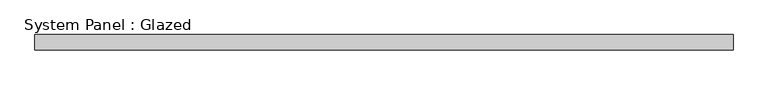
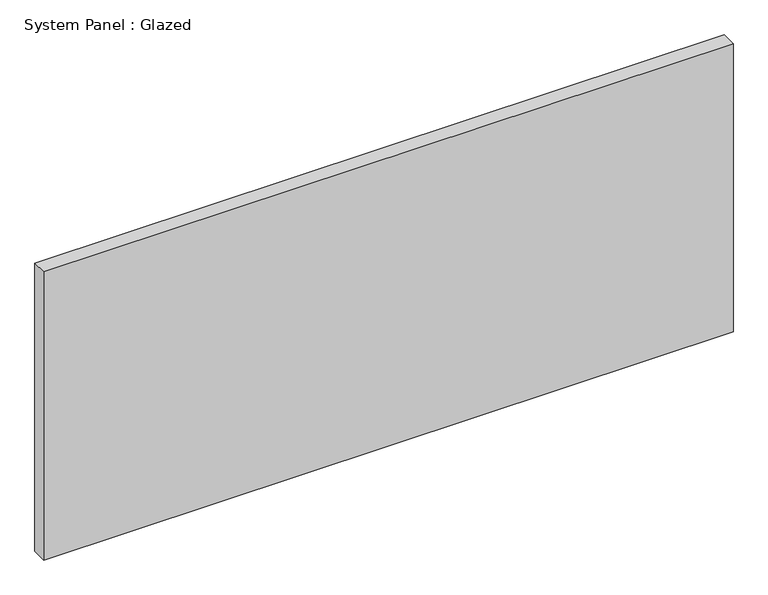
"""IFC4 building model written with IfcOpenShell, lengths in millimetres: plate geometry, System Panel : Glazed."""

from ifc_helpers import new_model, si_unit, origin, origin_with_axes, place, context, project, spatial, polyline, outline, extrude, source, transform, mapped, element, save


def system_panel_glazed_49ccfb91(model_context):
    return source(origin(), model_context, "Body", "SweptSolid", [
        extrude(outline(polyline([(582.0833333, 19.05), (-582.0833333, 19.05), (-582.0833333, 44.45), (582.0833333, 44.45), (582.0833333, 19.05)])), origin_with_axes(), (0.0, 0.0, 1.0), 514.35),
    ])


if __name__ == "__main__":
    model = new_model("IFC4")
    model_context = context("Model", 3, world=origin())
    ifc_project = project(units=[si_unit("LENGTHUNIT", "METRE", prefix="MILLI")], contexts=[model_context])
    site = spatial("IfcSite", under=ifc_project)
    building = spatial("IfcBuilding", under=site)
    placement = place(None, origin())
    system_panel_glazed_shape = system_panel_glazed_49ccfb91(model_context)
    element("IfcPlate", 1, ObjectType="System Panel : Glazed", at=placement, inside=building, context=model_context, shape_type="MappedRepresentation", body=[
        mapped(system_panel_glazed_shape, transform((0.0, 0.0, 0.0), x_axis=(1.0, 0.0, 0.0), y_axis=(0.0, 1.0, 0.0), z_axis=(0.0, 0.0, 1.0))),
    ])
    save(model, "model.ifc")

# Revit data of these elements
# Type "System Panel : Glazed"
#   Construction Type Id = "GSP4R"
#   Analytic Construction = "1/8 in Pilkington single glazing"
#   Visual Light Transmittance = 0.9
#   Solar Heat Gain Coefficient = 0.86
#   Heat Transfer Coefficient (U) = 1.18115 BTU/(h·ft²·°F)
# Element 1 (IfcPlate, "System Panel : Glazed")
#   Materials on its faces: "Glass"
# Materials
#   "Glass": class "Glass", colour RGB 0 128 192, transparency 0.75, Description = "Soda Lime Glass", Cost = 0
